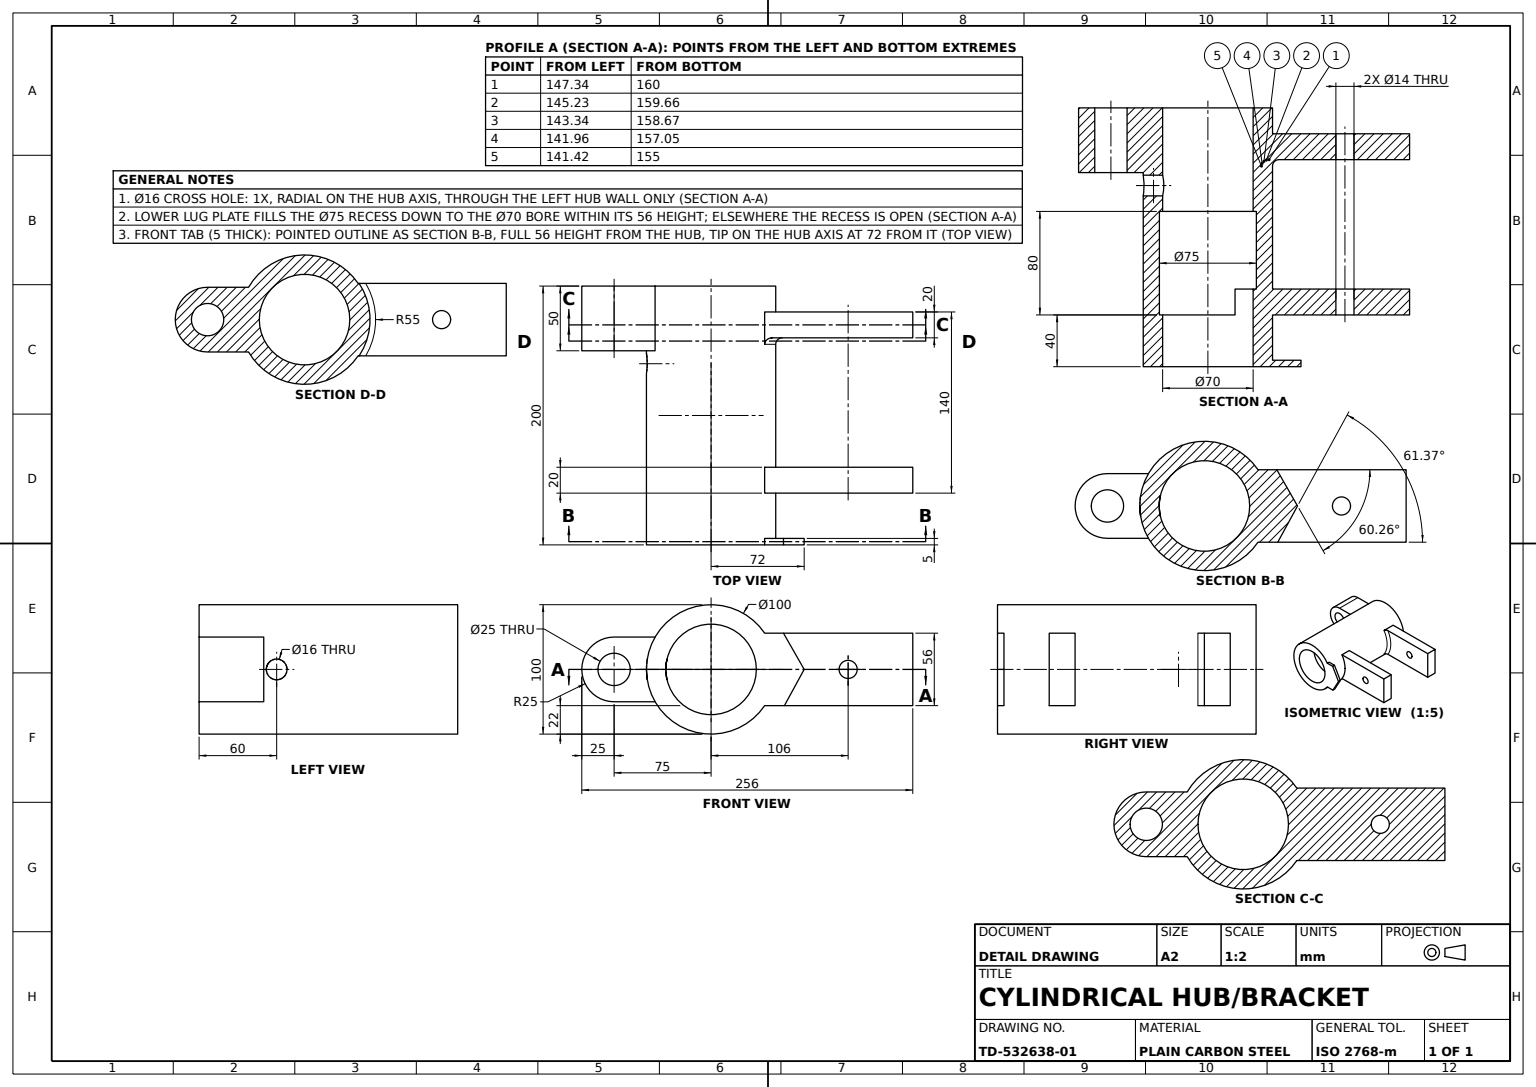
from build123d import *

# Parameters (mm, degrees)
BODY_PROFILE_100_R         = 50
HOUSING_BODY_100X200_DEPTH = 200
FRONT_BORE_PROFILE_70_R    = 35
FRONT_BORE_70X40_DEPTH     = 40
INNER_RECESS_PROFILE_75_R  = 37.5
INNER_RECESS_75X80_DEPTH   = 80
THROUGH_BORE_PROFILE_70_R  = 35
THROUGH_BORE_70_DEPTH      = 213.132034356
REAR_START                 = -5
REAR_TAB_5MM_DEPTH         = 5
LUG_PLATES_DEPTH           = 20
LUG_WEB_PROFILE_W          = 114.575369646
LUG_WEB_PROFILE_H          = 56
LUG_WEB_DEPTH              = 20
LUG_PIN_HOLES_PROFILE_14_R = 7
LUG_PIN_HOLES_14_DEPTH     = 229.989082709
LUG_WEB_FILLET_R5_R        = 5
TOP_BOSS_PROFILE_R         = 12.5
TOP_BOSS_DEPTH             = 50
TOP_BOSS_HOLE_PROFILE_16_R = 8
TOP_BOSS_HOLE_16_DEPTH     = 50


with BuildPart() as part:
    # Body Profile Ø100 → Housing Body Ø100x200 (new body)
    with BuildSketch(Plane.XY):
        Circle(BODY_PROFILE_100_R)
    extrude(amount=HOUSING_BODY_100X200_DEPTH)

    # Front Bore Profile Ø70 → Front Bore Ø70x40 (cut)
    with BuildSketch(Plane.XY.offset(200)):
        Circle(FRONT_BORE_PROFILE_70_R)
    extrude(amount=-FRONT_BORE_70X40_DEPTH, mode=Mode.SUBTRACT)

    # Inner Recess Profile Ø75 → Inner Recess Ø75x80 (cut)
    with BuildSketch(Plane.XY.offset(160)):
        Circle(INNER_RECESS_PROFILE_75_R)
    extrude(amount=-INNER_RECESS_75X80_DEPTH, mode=Mode.SUBTRACT)

    # Through Bore Profile Ø70 → Through Bore Ø70 (cut, through all)
    with BuildSketch(Plane(origin=(0, 0, 0), x_dir=(-1, 0, 0), z_dir=(0, 0, -1))):
        with Locations(Location((0, 0, 0), (0, 0, 180))):
            Circle(THROUGH_BORE_PROFILE_70_R)
    extrude(amount=-THROUGH_BORE_70_DEPTH, mode=Mode.SUBTRACT)

    # Rear Tab Profile → Rear Tab 5mm (add)
    with BuildSketch(Plane.XY.offset(200).offset(REAR_START)):
        with BuildLine():
            Line((72, 0), (56, 28))
            Line((56, 28), (41.424630354, 28))
            ThreePointArc((41.424630354, 28), (50, 0), (41.424630354, -28))
            Line((41.424630354, -28), (56.712315177, -28))
            Line((56.712315177, -28), (72, 0))
        make_face()
    extrude(amount=REAR_TAB_5MM_DEPTH)

    # Lug Plates Profile → Lug Plates (add)
    with BuildSketch(Plane.XY.offset(140)):
        with BuildLine():
            Line((21, -28), (156, -28))
            Line((156, -28), (156, 28))
            Line((156, 28), (21, 28))
            ThreePointArc((21, 28), (35, 0), (21, -28))
        make_face()
    extrude(amount=LUG_PLATES_DEPTH)

    # Lug Web Profile → Lug Web (add)
    with BuildSketch(Plane.XY.offset(20)):
        with Locations((98.712315177, 0)):
            Rectangle(LUG_WEB_PROFILE_W, LUG_WEB_PROFILE_H)
    extrude(amount=LUG_WEB_DEPTH)

    # Lug Pin Holes Profile Ø14 → Lug Pin Holes Ø14 (cut, through all)
    with BuildSketch(Plane.XY.offset(160)):
        with Locations(Location((106, 0, 0), (0, 0, 180))):
            Circle(LUG_PIN_HOLES_PROFILE_14_R)
    extrude(amount=-LUG_PIN_HOLES_14_DEPTH, mode=Mode.SUBTRACT)

    # Lug Web Fillet R5
    lug_web_fillet_r5_edges = [part.edges().sort_by_distance(p)[0] for p in [
        (47.808113944, -14.64186604, 40),
    ]]
    fillet(lug_web_fillet_r5_edges, radius=LUG_WEB_FILLET_R5_R)

    # Top Boss Profile → Top Boss (add)
    with BuildSketch(Plane.XY):
        with BuildLine():
            Line((-75, 25), (-43.301270189, 25))
            ThreePointArc((-43.301270189, 25), (-50, 0), (-43.301270189, -25))
            Line((-43.301270189, -25), (-75, -25))
            ThreePointArc((-75, -25), (-100, 0), (-75, 25))
        make_face()
        with Locations((-75, 0)):
            Circle(TOP_BOSS_PROFILE_R, mode=Mode.SUBTRACT)
    extrude(amount=TOP_BOSS_DEPTH)

    # Top Boss Hole Profile Ø16 → Top Boss Hole Ø16 (cut)
    with BuildSketch(Plane(origin=(-50, 0, 0), x_dir=(0, 0, -1), z_dir=(1, 0, 0))):
        with Locations(Location((-60, 0, 0), (0, 0, 180))):
            Circle(TOP_BOSS_HOLE_PROFILE_16_R)
    extrude(amount=TOP_BOSS_HOLE_16_DEPTH, mode=Mode.SUBTRACT)


solid = part.part
